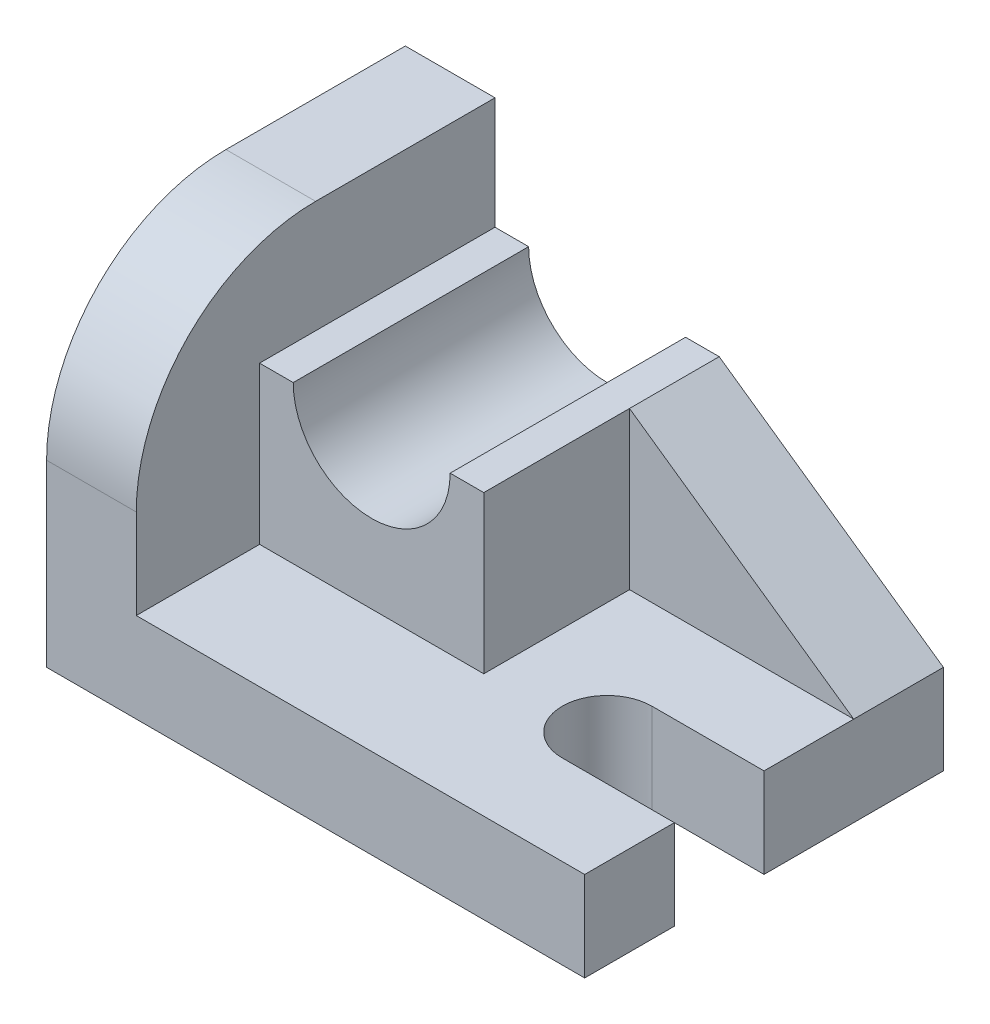
ISO-10303-21;
HEADER;
FILE_DESCRIPTION(('STEP AP214'),'2;1');
FILE_NAME('part.step','',(''),(''),'','','');
FILE_SCHEMA(('AUTOMOTIVE_DESIGN { 1 0 10303 214 1 1 1 1 }'));
ENDSEC;
DATA;
#1=APPLICATION_CONTEXT('core data for automotive mechanical design processes');
#2=APPLICATION_PROTOCOL_DEFINITION('international standard','automotive_design',2000,#1);
#3=PRODUCT_CONTEXT('',#1,'mechanical');
#4=PRODUCT('Part','Part','',(#3));
#5=PRODUCT_RELATED_PRODUCT_CATEGORY('part','',(#4));
#6=PRODUCT_DEFINITION_FORMATION('','',#4);
#7=PRODUCT_DEFINITION_CONTEXT('part definition',#1,'design');
#8=PRODUCT_DEFINITION('design','',#6,#7);
#9=PRODUCT_DEFINITION_SHAPE('','',#8);
#10=(LENGTH_UNIT() NAMED_UNIT(*) SI_UNIT(.MILLI.,.METRE.));
#11=(NAMED_UNIT(*) PLANE_ANGLE_UNIT() SI_UNIT($,.RADIAN.));
#12=(NAMED_UNIT(*) SI_UNIT($,.STERADIAN.) SOLID_ANGLE_UNIT());
#13=UNCERTAINTY_MEASURE_WITH_UNIT(LENGTH_MEASURE(1.E-05),#10,'distance_accuracy_value','');
#14=(GEOMETRIC_REPRESENTATION_CONTEXT(3) GLOBAL_UNCERTAINTY_ASSIGNED_CONTEXT((#13)) GLOBAL_UNIT_ASSIGNED_CONTEXT((#10,
#11,#12)) REPRESENTATION_CONTEXT('',''));
#15=CARTESIAN_POINT('',(0.,0.,0.));
#16=DIRECTION('',(0.,0.,1.));
#17=DIRECTION('',(1.,0.,0.));
#18=AXIS2_PLACEMENT_3D('',#15,#16,#17);
#19=CARTESIAN_POINT('',(0.,44.,0.));
#20=DIRECTION('',(0.,1.,0.));
#21=DIRECTION('',(0.,0.,1.));
#22=AXIS2_PLACEMENT_3D('',#19,#20,#21);
#23=PLANE('',#22);
#24=DIRECTION('',(0.,0.,1.));
#25=VECTOR('',#24,1.);
#26=CARTESIAN_POINT('',(22.,44.,-64.));
#27=LINE('',#26,#25);
#28=CARTESIAN_POINT('',(22.,44.,-64.));
#29=VERTEX_POINT('',#28);
#30=CARTESIAN_POINT('',(22.,44.,-22.));
#31=VERTEX_POINT('',#30);
#32=EDGE_CURVE('E11',#29,#31,#27,.T.);
#33=ORIENTED_EDGE('',*,*,#32,.F.);
#34=DIRECTION('',(-1.,0.,0.));
#35=VECTOR('',#34,1.);
#36=CARTESIAN_POINT('',(16.,44.,-64.));
#37=LINE('',#36,#35);
#38=CARTESIAN_POINT('',(16.,44.,-64.));
#39=VERTEX_POINT('',#38);
#40=EDGE_CURVE('E226',#29,#39,#37,.T.);
#41=ORIENTED_EDGE('',*,*,#40,.T.);
#42=DIRECTION('',(0.,0.,1.));
#43=VECTOR('',#42,1.);
#44=CARTESIAN_POINT('',(16.,44.,-64.));
#45=LINE('',#44,#43);
#46=CARTESIAN_POINT('',(16.,44.,-22.));
#47=VERTEX_POINT('',#46);
#48=EDGE_CURVE('E241',#39,#47,#45,.T.);
#49=ORIENTED_EDGE('',*,*,#48,.T.);
#50=DIRECTION('',(1.,0.,0.));
#51=VECTOR('',#50,1.);
#52=CARTESIAN_POINT('',(16.,44.,-22.));
#53=LINE('',#52,#51);
#54=EDGE_CURVE('E325',#47,#31,#53,.T.);
#55=ORIENTED_EDGE('',*,*,#54,.T.);
#56=EDGE_LOOP('',(#33,#41,#49,#55));
#57=FACE_BOUND('',#56,.T.);
#58=ADVANCED_FACE('F39',(#57),#23,.T.);
#59=CARTESIAN_POINT('',(0.,16.,0.));
#60=DIRECTION('',(0.,-1.,0.));
#61=DIRECTION('',(0.,0.,-1.));
#62=AXIS2_PLACEMENT_3D('',#59,#60,#61);
#63=PLANE('',#62);
#64=DIRECTION('',(0.,0.,-1.));
#65=VECTOR('',#64,1.);
#66=CARTESIAN_POINT('',(96.,16.,0.));
#67=LINE('',#66,#65);
#68=CARTESIAN_POINT('',(96.,16.,-32.));
#69=VERTEX_POINT('',#68);
#70=CARTESIAN_POINT('',(96.,16.,-48.));
#71=VERTEX_POINT('',#70);
#72=EDGE_CURVE('E180',#69,#71,#67,.T.);
#73=ORIENTED_EDGE('',*,*,#72,.T.);
#74=DIRECTION('',(-1.,0.,0.));
#75=VECTOR('',#74,1.);
#76=CARTESIAN_POINT('',(56.,16.,-48.));
#77=LINE('',#76,#75);
#78=CARTESIAN_POINT('',(56.,16.,-48.));
#79=VERTEX_POINT('',#78);
#80=EDGE_CURVE('E160',#71,#79,#77,.T.);
#81=ORIENTED_EDGE('',*,*,#80,.T.);
#82=DIRECTION('',(0.,0.,-1.));
#83=VECTOR('',#82,1.);
#84=CARTESIAN_POINT('',(56.,16.,-64.));
#85=LINE('',#84,#83);
#86=CARTESIAN_POINT('',(56.,16.,-22.));
#87=VERTEX_POINT('',#86);
#88=EDGE_CURVE('E62',#87,#79,#85,.T.);
#89=ORIENTED_EDGE('',*,*,#88,.F.);
#90=DIRECTION('',(1.,0.,0.));
#91=VECTOR('',#90,1.);
#92=CARTESIAN_POINT('',(16.,16.,-22.));
#93=LINE('',#92,#91);
#94=CARTESIAN_POINT('',(16.,16.,-22.));
#95=VERTEX_POINT('',#94);
#96=EDGE_CURVE('E228',#95,#87,#93,.T.);
#97=ORIENTED_EDGE('',*,*,#96,.F.);
#98=DIRECTION('',(0.,0.,1.));
#99=VECTOR('',#98,1.);
#100=CARTESIAN_POINT('',(16.,16.,0.));
#101=LINE('',#100,#99);
#102=CARTESIAN_POINT('',(16.,16.,0.));
#103=VERTEX_POINT('',#102);
#104=EDGE_CURVE('E268',#95,#103,#101,.T.);
#105=ORIENTED_EDGE('',*,*,#104,.T.);
#106=DIRECTION('',(1.,0.,0.));
#107=VECTOR('',#106,1.);
#108=CARTESIAN_POINT('',(0.,16.,0.));
#109=LINE('',#108,#107);
#110=CARTESIAN_POINT('',(96.,16.,0.));
#111=VERTEX_POINT('',#110);
#112=EDGE_CURVE('E186',#103,#111,#109,.T.);
#113=ORIENTED_EDGE('',*,*,#112,.T.);
#114=CARTESIAN_POINT('',(96.,16.,-16.));
#115=VERTEX_POINT('',#114);
#116=EDGE_CURVE('E190',#111,#115,#67,.T.);
#117=ORIENTED_EDGE('',*,*,#116,.T.);
#118=DIRECTION('',(1.,0.,0.));
#119=VECTOR('',#118,1.);
#120=CARTESIAN_POINT('',(96.,16.,-16.));
#121=LINE('',#120,#119);
#122=CARTESIAN_POINT('',(76.,16.,-16.));
#123=VERTEX_POINT('',#122);
#124=EDGE_CURVE('E279',#123,#115,#121,.T.);
#125=ORIENTED_EDGE('',*,*,#124,.F.);
#126=CARTESIAN_POINT('',(76.,16.,-24.));
#127=DIRECTION('',(0.,1.,0.));
#128=DIRECTION('',(0.,0.,1.));
#129=AXIS2_PLACEMENT_3D('',#126,#127,#128);
#130=CIRCLE('',#129,8.);
#131=CARTESIAN_POINT('',(76.,16.,-32.));
#132=VERTEX_POINT('',#131);
#133=EDGE_CURVE('E288',#132,#123,#130,.T.);
#134=ORIENTED_EDGE('',*,*,#133,.F.);
#135=DIRECTION('',(-1.,0.,0.));
#136=VECTOR('',#135,1.);
#137=CARTESIAN_POINT('',(96.,16.,-32.));
#138=LINE('',#137,#136);
#139=EDGE_CURVE('E189',#69,#132,#138,.T.);
#140=ORIENTED_EDGE('',*,*,#139,.F.);
#141=EDGE_LOOP('',(#73,#81,#89,#97,#105,#113,#117,#125,#134,#140));
#142=FACE_BOUND('',#141,.T.);
#143=ADVANCED_FACE('F184',(#142),#63,.F.);
#144=CARTESIAN_POINT('',(16.,32.,-32.));
#145=DIRECTION('',(1.,0.,0.));
#146=DIRECTION('',(0.,0.,-1.));
#147=AXIS2_PLACEMENT_3D('',#144,#145,#146);
#148=PLANE('',#147);
#149=ORIENTED_EDGE('',*,*,#104,.F.);
#150=DIRECTION('',(0.,-1.,0.));
#151=VECTOR('',#150,1.);
#152=CARTESIAN_POINT('',(16.,44.,-22.));
#153=LINE('',#152,#151);
#154=EDGE_CURVE('E240',#47,#95,#153,.T.);
#155=ORIENTED_EDGE('',*,*,#154,.F.);
#156=ORIENTED_EDGE('',*,*,#48,.F.);
#157=DIRECTION('',(0.,-1.,0.));
#158=VECTOR('',#157,1.);
#159=CARTESIAN_POINT('',(16.,0.,-64.));
#160=LINE('',#159,#158);
#161=CARTESIAN_POINT('',(16.,64.,-64.));
#162=VERTEX_POINT('',#161);
#163=EDGE_CURVE('E250',#162,#39,#160,.T.);
#164=ORIENTED_EDGE('',*,*,#163,.F.);
#165=DIRECTION('',(0.,0.,-1.));
#166=VECTOR('',#165,1.);
#167=CARTESIAN_POINT('',(16.,64.,-64.));
#168=LINE('',#167,#166);
#169=CARTESIAN_POINT('',(16.,64.,-32.0000000000002));
#170=VERTEX_POINT('',#169);
#171=EDGE_CURVE('E260',#170,#162,#168,.T.);
#172=ORIENTED_EDGE('',*,*,#171,.F.);
#173=CARTESIAN_POINT('',(16.,32.,-32.));
#174=DIRECTION('',(-1.,0.,0.));
#175=DIRECTION('',(0.,0.,-1.));
#176=AXIS2_PLACEMENT_3D('',#173,#174,#175);
#177=CIRCLE('',#176,32.);
#178=CARTESIAN_POINT('',(16.,31.9999999999998,0.));
#179=VERTEX_POINT('',#178);
#180=EDGE_CURVE('E255',#179,#170,#177,.T.);
#181=ORIENTED_EDGE('',*,*,#180,.F.);
#182=DIRECTION('',(0.,1.,0.));
#183=VECTOR('',#182,1.);
#184=CARTESIAN_POINT('',(16.,0.,0.));
#185=LINE('',#184,#183);
#186=EDGE_CURVE('E253',#103,#179,#185,.T.);
#187=ORIENTED_EDGE('',*,*,#186,.F.);
#188=EDGE_LOOP('',(#149,#155,#156,#164,#172,#181,#187));
#189=FACE_BOUND('',#188,.T.);
#190=ADVANCED_FACE('F314',(#189),#148,.T.);
#191=CARTESIAN_POINT('',(96.,16.,0.));
#192=DIRECTION('',(-1.,0.,0.));
#193=DIRECTION('',(0.,0.,1.));
#194=AXIS2_PLACEMENT_3D('',#191,#192,#193);
#195=PLANE('',#194);
#196=DIRECTION('',(0.,0.,-1.));
#197=VECTOR('',#196,1.);
#198=CARTESIAN_POINT('',(96.,0.,0.));
#199=LINE('',#198,#197);
#200=CARTESIAN_POINT('',(96.,0.,0.));
#201=VERTEX_POINT('',#200);
#202=CARTESIAN_POINT('',(96.,0.,-16.));
#203=VERTEX_POINT('',#202);
#204=EDGE_CURVE('E204',#201,#203,#199,.T.);
#205=ORIENTED_EDGE('',*,*,#204,.T.);
#206=DIRECTION('',(0.,1.,0.));
#207=VECTOR('',#206,1.);
#208=CARTESIAN_POINT('',(96.,0.,-16.));
#209=LINE('',#208,#207);
#210=EDGE_CURVE('E203',#203,#115,#209,.T.);
#211=ORIENTED_EDGE('',*,*,#210,.T.);
#212=ORIENTED_EDGE('',*,*,#116,.F.);
#213=DIRECTION('',(0.,-1.,0.));
#214=VECTOR('',#213,1.);
#215=CARTESIAN_POINT('',(96.,16.,0.));
#216=LINE('',#215,#214);
#217=EDGE_CURVE('E211',#111,#201,#216,.T.);
#218=ORIENTED_EDGE('',*,*,#217,.T.);
#219=EDGE_LOOP('',(#205,#211,#212,#218));
#220=FACE_BOUND('',#219,.T.);
#221=ADVANCED_FACE('F369',(#220),#195,.F.);
#222=CARTESIAN_POINT('',(0.,16.,0.));
#223=DIRECTION('',(1.,0.,0.));
#224=DIRECTION('',(0.,0.,-1.));
#225=AXIS2_PLACEMENT_3D('',#222,#223,#224);
#226=PLANE('',#225);
#227=DIRECTION('',(0.,0.,1.));
#228=VECTOR('',#227,1.);
#229=CARTESIAN_POINT('',(0.,0.,0.));
#230=LINE('',#229,#228);
#231=CARTESIAN_POINT('',(0.,0.,-64.));
#232=VERTEX_POINT('',#231);
#233=CARTESIAN_POINT('',(0.,0.,0.));
#234=VERTEX_POINT('',#233);
#235=EDGE_CURVE('E197',#232,#234,#230,.T.);
#236=ORIENTED_EDGE('',*,*,#235,.T.);
#237=DIRECTION('',(0.,-1.,0.));
#238=VECTOR('',#237,1.);
#239=CARTESIAN_POINT('',(0.,16.,0.));
#240=LINE('',#239,#238);
#241=CARTESIAN_POINT('',(0.,31.9999999999998,0.));
#242=VERTEX_POINT('',#241);
#243=EDGE_CURVE('E212',#242,#234,#240,.T.);
#244=ORIENTED_EDGE('',*,*,#243,.F.);
#245=CARTESIAN_POINT('',(0.,32.,-32.));
#246=DIRECTION('',(-1.,0.,0.));
#247=DIRECTION('',(0.,0.,-1.));
#248=AXIS2_PLACEMENT_3D('',#245,#246,#247);
#249=CIRCLE('',#248,32.);
#250=CARTESIAN_POINT('',(0.,64.,-32.0000000000002));
#251=VERTEX_POINT('',#250);
#252=EDGE_CURVE('E247',#242,#251,#249,.T.);
#253=ORIENTED_EDGE('',*,*,#252,.T.);
#254=DIRECTION('',(0.,0.,-1.));
#255=VECTOR('',#254,1.);
#256=CARTESIAN_POINT('',(0.,64.,-64.));
#257=LINE('',#256,#255);
#258=CARTESIAN_POINT('',(0.,64.,-64.));
#259=VERTEX_POINT('',#258);
#260=EDGE_CURVE('E252',#251,#259,#257,.T.);
#261=ORIENTED_EDGE('',*,*,#260,.T.);
#262=DIRECTION('',(0.,-1.,0.));
#263=VECTOR('',#262,1.);
#264=CARTESIAN_POINT('',(0.,16.,-64.));
#265=LINE('',#264,#263);
#266=EDGE_CURVE('E194',#259,#232,#265,.T.);
#267=ORIENTED_EDGE('',*,*,#266,.T.);
#268=EDGE_LOOP('',(#236,#244,#253,#261,#267));
#269=FACE_BOUND('',#268,.T.);
#270=ADVANCED_FACE('F41',(#269),#226,.F.);
#271=CARTESIAN_POINT('',(0.,16.,0.));
#272=DIRECTION('',(0.,0.,-1.));
#273=DIRECTION('',(-1.,0.,0.));
#274=AXIS2_PLACEMENT_3D('',#271,#272,#273);
#275=PLANE('',#274);
#276=ORIENTED_EDGE('',*,*,#112,.F.);
#277=ORIENTED_EDGE('',*,*,#186,.T.);
#278=DIRECTION('',(-1.,0.,0.));
#279=VECTOR('',#278,1.);
#280=CARTESIAN_POINT('',(16.,31.9999999999998,0.));
#281=LINE('',#280,#279);
#282=EDGE_CURVE('E257',#179,#242,#281,.T.);
#283=ORIENTED_EDGE('',*,*,#282,.T.);
#284=ORIENTED_EDGE('',*,*,#243,.T.);
#285=DIRECTION('',(1.,0.,0.));
#286=VECTOR('',#285,1.);
#287=CARTESIAN_POINT('',(0.,0.,0.));
#288=LINE('',#287,#286);
#289=EDGE_CURVE('E199',#234,#201,#288,.T.);
#290=ORIENTED_EDGE('',*,*,#289,.T.);
#291=ORIENTED_EDGE('',*,*,#217,.F.);
#292=EDGE_LOOP('',(#276,#277,#283,#284,#290,#291));
#293=FACE_BOUND('',#292,.T.);
#294=ADVANCED_FACE('F339',(#293),#275,.F.);
#295=ORIENTED_EDGE('',*,*,#72,.F.);
#296=DIRECTION('',(0.,1.,0.));
#297=VECTOR('',#296,1.);
#298=CARTESIAN_POINT('',(96.,0.,-32.));
#299=LINE('',#298,#297);
#300=CARTESIAN_POINT('',(96.,0.,-32.));
#301=VERTEX_POINT('',#300);
#302=EDGE_CURVE('E281',#301,#69,#299,.T.);
#303=ORIENTED_EDGE('',*,*,#302,.F.);
#304=CARTESIAN_POINT('',(96.,0.,-64.));
#305=VERTEX_POINT('',#304);
#306=EDGE_CURVE('E201',#301,#305,#199,.T.);
#307=ORIENTED_EDGE('',*,*,#306,.T.);
#308=DIRECTION('',(0.,-1.,0.));
#309=VECTOR('',#308,1.);
#310=CARTESIAN_POINT('',(96.,16.,-64.));
#311=LINE('',#310,#309);
#312=CARTESIAN_POINT('',(96.,16.,-64.));
#313=VERTEX_POINT('',#312);
#314=EDGE_CURVE('E182',#313,#305,#311,.T.);
#315=ORIENTED_EDGE('',*,*,#314,.F.);
#316=DIRECTION('',(0.,0.,-1.));
#317=VECTOR('',#316,1.);
#318=CARTESIAN_POINT('',(96.,16.,-48.));
#319=LINE('',#318,#317);
#320=EDGE_CURVE('E169',#71,#313,#319,.T.);
#321=ORIENTED_EDGE('',*,*,#320,.F.);
#322=EDGE_LOOP('',(#295,#303,#307,#315,#321));
#323=FACE_BOUND('',#322,.T.);
#324=ADVANCED_FACE('F179',(#323),#195,.F.);
#325=CARTESIAN_POINT('',(0.,16.,-64.));
#326=DIRECTION('',(0.,0.,1.));
#327=DIRECTION('',(1.,0.,0.));
#328=AXIS2_PLACEMENT_3D('',#325,#326,#327);
#329=PLANE('',#328);
#330=ORIENTED_EDGE('',*,*,#40,.F.);
#331=CARTESIAN_POINT('',(36.,44.,-64.));
#332=DIRECTION('',(0.,0.,1.));
#333=DIRECTION('',(1.,0.,0.));
#334=AXIS2_PLACEMENT_3D('',#331,#332,#333);
#335=CIRCLE('',#334,14.);
#336=CARTESIAN_POINT('',(50.,44.,-64.));
#337=VERTEX_POINT('',#336);
#338=EDGE_CURVE('E217',#29,#337,#335,.T.);
#339=ORIENTED_EDGE('',*,*,#338,.T.);
#340=CARTESIAN_POINT('',(56.,44.,-64.));
#341=VERTEX_POINT('',#340);
#342=EDGE_CURVE('E229',#341,#337,#37,.T.);
#343=ORIENTED_EDGE('',*,*,#342,.F.);
#344=DIRECTION('',(0.819231920519041,-0.573462344363328,0.));
#345=VECTOR('',#344,1.);
#346=CARTESIAN_POINT('',(96.,16.,-64.));
#347=LINE('',#346,#345);
#348=EDGE_CURVE('E174',#341,#313,#347,.T.);
#349=ORIENTED_EDGE('',*,*,#348,.T.);
#350=ORIENTED_EDGE('',*,*,#314,.T.);
#351=DIRECTION('',(-1.,0.,0.));
#352=VECTOR('',#351,1.);
#353=CARTESIAN_POINT('',(0.,0.,-64.));
#354=LINE('',#353,#352);
#355=EDGE_CURVE('E192',#305,#232,#354,.T.);
#356=ORIENTED_EDGE('',*,*,#355,.T.);
#357=ORIENTED_EDGE('',*,*,#266,.F.);
#358=DIRECTION('',(-1.,0.,0.));
#359=VECTOR('',#358,1.);
#360=CARTESIAN_POINT('',(16.,64.,-64.));
#361=LINE('',#360,#359);
#362=EDGE_CURVE('E264',#162,#259,#361,.T.);
#363=ORIENTED_EDGE('',*,*,#362,.F.);
#364=ORIENTED_EDGE('',*,*,#163,.T.);
#365=EDGE_LOOP('',(#330,#339,#343,#349,#350,#356,#357,#363,#364));
#366=FACE_BOUND('',#365,.T.);
#367=ADVANCED_FACE('F227',(#366),#329,.F.);
#368=CARTESIAN_POINT('',(0.,0.,0.));
#369=DIRECTION('',(0.,-1.,0.));
#370=DIRECTION('',(0.,0.,-1.));
#371=AXIS2_PLACEMENT_3D('',#368,#369,#370);
#372=PLANE('',#371);
#373=ORIENTED_EDGE('',*,*,#204,.F.);
#374=ORIENTED_EDGE('',*,*,#289,.F.);
#375=ORIENTED_EDGE('',*,*,#235,.F.);
#376=ORIENTED_EDGE('',*,*,#355,.F.);
#377=ORIENTED_EDGE('',*,*,#306,.F.);
#378=DIRECTION('',(-1.,0.,0.));
#379=VECTOR('',#378,1.);
#380=CARTESIAN_POINT('',(96.,0.,-32.));
#381=LINE('',#380,#379);
#382=CARTESIAN_POINT('',(76.,0.,-32.));
#383=VERTEX_POINT('',#382);
#384=EDGE_CURVE('E273',#301,#383,#381,.T.);
#385=ORIENTED_EDGE('',*,*,#384,.T.);
#386=CARTESIAN_POINT('',(76.,0.,-24.));
#387=DIRECTION('',(0.,1.,0.));
#388=DIRECTION('',(0.,0.,1.));
#389=AXIS2_PLACEMENT_3D('',#386,#387,#388);
#390=CIRCLE('',#389,8.);
#391=CARTESIAN_POINT('',(76.,0.,-16.));
#392=VERTEX_POINT('',#391);
#393=EDGE_CURVE('E280',#383,#392,#390,.T.);
#394=ORIENTED_EDGE('',*,*,#393,.T.);
#395=DIRECTION('',(1.,0.,0.));
#396=VECTOR('',#395,1.);
#397=CARTESIAN_POINT('',(96.,0.,-16.));
#398=LINE('',#397,#396);
#399=EDGE_CURVE('E282',#392,#203,#398,.T.);
#400=ORIENTED_EDGE('',*,*,#399,.T.);
#401=EDGE_LOOP('',(#373,#374,#375,#376,#377,#385,#394,#400));
#402=FACE_BOUND('',#401,.T.);
#403=ADVANCED_FACE('F304',(#402),#372,.T.);
#404=CARTESIAN_POINT('',(96.,0.,-16.));
#405=DIRECTION('',(0.,0.,1.));
#406=DIRECTION('',(1.,0.,0.));
#407=AXIS2_PLACEMENT_3D('',#404,#405,#406);
#408=PLANE('',#407);
#409=ORIENTED_EDGE('',*,*,#124,.T.);
#410=ORIENTED_EDGE('',*,*,#210,.F.);
#411=ORIENTED_EDGE('',*,*,#399,.F.);
#412=DIRECTION('',(0.,1.,0.));
#413=VECTOR('',#412,1.);
#414=CARTESIAN_POINT('',(76.,0.,-16.));
#415=LINE('',#414,#413);
#416=EDGE_CURVE('E295',#392,#123,#415,.T.);
#417=ORIENTED_EDGE('',*,*,#416,.T.);
#418=EDGE_LOOP('',(#409,#410,#411,#417));
#419=FACE_BOUND('',#418,.T.);
#420=ADVANCED_FACE('F398',(#419),#408,.F.);
#421=CARTESIAN_POINT('',(76.,0.,-24.));
#422=DIRECTION('',(0.,1.,0.));
#423=DIRECTION('',(0.,0.,1.));
#424=AXIS2_PLACEMENT_3D('',#421,#422,#423);
#425=CYLINDRICAL_SURFACE('',#424,8.);
#426=ORIENTED_EDGE('',*,*,#133,.T.);
#427=ORIENTED_EDGE('',*,*,#416,.F.);
#428=ORIENTED_EDGE('',*,*,#393,.F.);
#429=DIRECTION('',(0.,1.,0.));
#430=VECTOR('',#429,1.);
#431=CARTESIAN_POINT('',(76.,0.,-32.));
#432=LINE('',#431,#430);
#433=EDGE_CURVE('E294',#383,#132,#432,.T.);
#434=ORIENTED_EDGE('',*,*,#433,.T.);
#435=EDGE_LOOP('',(#426,#427,#428,#434));
#436=FACE_BOUND('',#435,.T.);
#437=ADVANCED_FACE('F494',(#436),#425,.F.);
#438=CARTESIAN_POINT('',(96.,0.,-32.));
#439=DIRECTION('',(0.,0.,-1.));
#440=DIRECTION('',(-1.,0.,0.));
#441=AXIS2_PLACEMENT_3D('',#438,#439,#440);
#442=PLANE('',#441);
#443=ORIENTED_EDGE('',*,*,#139,.T.);
#444=ORIENTED_EDGE('',*,*,#433,.F.);
#445=ORIENTED_EDGE('',*,*,#384,.F.);
#446=ORIENTED_EDGE('',*,*,#302,.T.);
#447=EDGE_LOOP('',(#443,#444,#445,#446));
#448=FACE_BOUND('',#447,.T.);
#449=ADVANCED_FACE('F297',(#448),#442,.F.);
#450=CARTESIAN_POINT('',(16.,64.,-64.));
#451=DIRECTION('',(0.,1.,0.));
#452=DIRECTION('',(0.,0.,1.));
#453=AXIS2_PLACEMENT_3D('',#450,#451,#452);
#454=PLANE('',#453);
#455=ORIENTED_EDGE('',*,*,#260,.F.);
#456=DIRECTION('',(-1.,0.,0.));
#457=VECTOR('',#456,1.);
#458=CARTESIAN_POINT('',(16.,64.,-32.0000000000002));
#459=LINE('',#458,#457);
#460=EDGE_CURVE('E267',#170,#251,#459,.T.);
#461=ORIENTED_EDGE('',*,*,#460,.F.);
#462=ORIENTED_EDGE('',*,*,#171,.T.);
#463=ORIENTED_EDGE('',*,*,#362,.T.);
#464=EDGE_LOOP('',(#455,#461,#462,#463));
#465=FACE_BOUND('',#464,.T.);
#466=ADVANCED_FACE('F306',(#465),#454,.T.);
#467=CARTESIAN_POINT('',(16.,32.,-32.));
#468=DIRECTION('',(-1.,0.,0.));
#469=DIRECTION('',(0.,0.,1.));
#470=AXIS2_PLACEMENT_3D('',#467,#468,#469);
#471=CYLINDRICAL_SURFACE('',#470,32.);
#472=ORIENTED_EDGE('',*,*,#252,.F.);
#473=ORIENTED_EDGE('',*,*,#282,.F.);
#474=ORIENTED_EDGE('',*,*,#180,.T.);
#475=ORIENTED_EDGE('',*,*,#460,.T.);
#476=EDGE_LOOP('',(#472,#473,#474,#475));
#477=FACE_BOUND('',#476,.T.);
#478=ADVANCED_FACE('F338',(#477),#471,.T.);
#479=CARTESIAN_POINT('',(16.,44.,-22.));
#480=DIRECTION('',(0.,0.,-1.));
#481=DIRECTION('',(-1.,0.,0.));
#482=AXIS2_PLACEMENT_3D('',#479,#480,#481);
#483=PLANE('',#482);
#484=CARTESIAN_POINT('',(50.,44.,-22.));
#485=VERTEX_POINT('',#484);
#486=CARTESIAN_POINT('',(56.,44.,-22.));
#487=VERTEX_POINT('',#486);
#488=EDGE_CURVE('E319',#485,#487,#53,.T.);
#489=ORIENTED_EDGE('',*,*,#488,.F.);
#490=CARTESIAN_POINT('',(36.,44.,-22.));
#491=DIRECTION('',(0.,0.,1.));
#492=DIRECTION('',(1.,0.,0.));
#493=AXIS2_PLACEMENT_3D('',#490,#491,#492);
#494=CIRCLE('',#493,14.);
#495=EDGE_CURVE('E52',#31,#485,#494,.T.);
#496=ORIENTED_EDGE('',*,*,#495,.F.);
#497=ORIENTED_EDGE('',*,*,#54,.F.);
#498=ORIENTED_EDGE('',*,*,#154,.T.);
#499=ORIENTED_EDGE('',*,*,#96,.T.);
#500=DIRECTION('',(0.,-1.,0.));
#501=VECTOR('',#500,1.);
#502=CARTESIAN_POINT('',(56.,44.,-22.));
#503=LINE('',#502,#501);
#504=EDGE_CURVE('E235',#487,#87,#503,.T.);
#505=ORIENTED_EDGE('',*,*,#504,.F.);
#506=EDGE_LOOP('',(#489,#496,#497,#498,#499,#505));
#507=FACE_BOUND('',#506,.T.);
#508=ADVANCED_FACE('F335',(#507),#483,.F.);
#509=CARTESIAN_POINT('',(56.,44.,-64.));
#510=DIRECTION('',(-1.,0.,0.));
#511=DIRECTION('',(0.,0.,1.));
#512=AXIS2_PLACEMENT_3D('',#509,#510,#511);
#513=PLANE('',#512);
#514=ORIENTED_EDGE('',*,*,#88,.T.);
#515=DIRECTION('',(0.,1.,0.));
#516=VECTOR('',#515,1.);
#517=CARTESIAN_POINT('',(56.,44.,-48.));
#518=LINE('',#517,#516);
#519=CARTESIAN_POINT('',(56.,44.,-48.));
#520=VERTEX_POINT('',#519);
#521=EDGE_CURVE('E165',#79,#520,#518,.T.);
#522=ORIENTED_EDGE('',*,*,#521,.T.);
#523=DIRECTION('',(0.,0.,-1.));
#524=VECTOR('',#523,1.);
#525=CARTESIAN_POINT('',(56.,44.,-64.));
#526=LINE('',#525,#524);
#527=EDGE_CURVE('E239',#487,#520,#526,.T.);
#528=ORIENTED_EDGE('',*,*,#527,.F.);
#529=ORIENTED_EDGE('',*,*,#504,.T.);
#530=EDGE_LOOP('',(#514,#522,#528,#529));
#531=FACE_BOUND('',#530,.T.);
#532=ADVANCED_FACE('F330',(#531),#513,.F.);
#533=DIRECTION('',(0.,0.,1.));
#534=VECTOR('',#533,1.);
#535=CARTESIAN_POINT('',(50.,44.,-64.));
#536=LINE('',#535,#534);
#537=EDGE_CURVE('E50',#485,#337,#536,.F.);
#538=ORIENTED_EDGE('',*,*,#537,.F.);
#539=ORIENTED_EDGE('',*,*,#488,.T.);
#540=ORIENTED_EDGE('',*,*,#527,.T.);
#541=DIRECTION('',(0.,0.,-1.));
#542=VECTOR('',#541,1.);
#543=CARTESIAN_POINT('',(56.,44.,-48.));
#544=LINE('',#543,#542);
#545=EDGE_CURVE('E172',#520,#341,#544,.T.);
#546=ORIENTED_EDGE('',*,*,#545,.T.);
#547=ORIENTED_EDGE('',*,*,#342,.T.);
#548=EDGE_LOOP('',(#538,#539,#540,#546,#547));
#549=FACE_BOUND('',#548,.T.);
#550=ADVANCED_FACE('F234',(#549),#23,.T.);
#551=CARTESIAN_POINT('',(36.,44.,-64.));
#552=DIRECTION('',(0.,0.,1.));
#553=DIRECTION('',(1.,0.,0.));
#554=AXIS2_PLACEMENT_3D('',#551,#552,#553);
#555=CYLINDRICAL_SURFACE('',#554,14.);
#556=ORIENTED_EDGE('',*,*,#32,.T.);
#557=ORIENTED_EDGE('',*,*,#495,.T.);
#558=ORIENTED_EDGE('',*,*,#537,.T.);
#559=ORIENTED_EDGE('',*,*,#338,.F.);
#560=EDGE_LOOP('',(#556,#557,#558,#559));
#561=FACE_BOUND('',#560,.T.);
#562=ADVANCED_FACE('F220',(#561),#555,.F.);
#563=CARTESIAN_POINT('',(96.,16.,-48.));
#564=DIRECTION('',(0.573462344363328,0.819231920519041,0.));
#565=DIRECTION('',(-0.819231920519041,0.573462344363328,0.));
#566=AXIS2_PLACEMENT_3D('',#563,#564,#565);
#567=PLANE('',#566);
#568=ORIENTED_EDGE('',*,*,#348,.F.);
#569=ORIENTED_EDGE('',*,*,#545,.F.);
#570=DIRECTION('',(0.819231920519041,-0.573462344363328,0.));
#571=VECTOR('',#570,1.);
#572=CARTESIAN_POINT('',(96.,16.,-48.));
#573=LINE('',#572,#571);
#574=EDGE_CURVE('E159',#520,#71,#573,.T.);
#575=ORIENTED_EDGE('',*,*,#574,.T.);
#576=ORIENTED_EDGE('',*,*,#320,.T.);
#577=EDGE_LOOP('',(#568,#569,#575,#576));
#578=FACE_BOUND('',#577,.T.);
#579=ADVANCED_FACE('F170',(#578),#567,.T.);
#580=CARTESIAN_POINT('',(0.,0.,-48.));
#581=DIRECTION('',(0.,0.,1.));
#582=DIRECTION('',(1.,0.,0.));
#583=AXIS2_PLACEMENT_3D('',#580,#581,#582);
#584=PLANE('',#583);
#585=ORIENTED_EDGE('',*,*,#574,.F.);
#586=ORIENTED_EDGE('',*,*,#521,.F.);
#587=ORIENTED_EDGE('',*,*,#80,.F.);
#588=EDGE_LOOP('',(#585,#586,#587));
#589=FACE_BOUND('',#588,.T.);
#590=ADVANCED_FACE('F157',(#589),#584,.T.);
#591=CLOSED_SHELL('',(#58,#143,#190,#221,#270,#294,#324,#367,#403,#420,#437,#449,#466,#478,#508,
#532,#550,#562,#579,#590));
#592=MANIFOLD_SOLID_BREP('B2',#591);
#593=ADVANCED_BREP_SHAPE_REPRESENTATION('',(#18,#592),#14);
#594=SHAPE_DEFINITION_REPRESENTATION(#9,#593);
ENDSEC;
END-ISO-10303-21;
